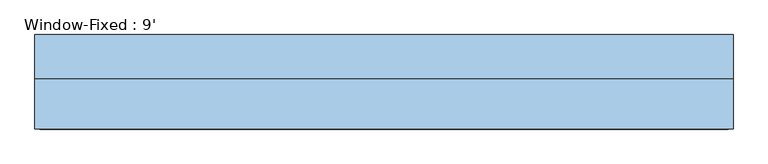
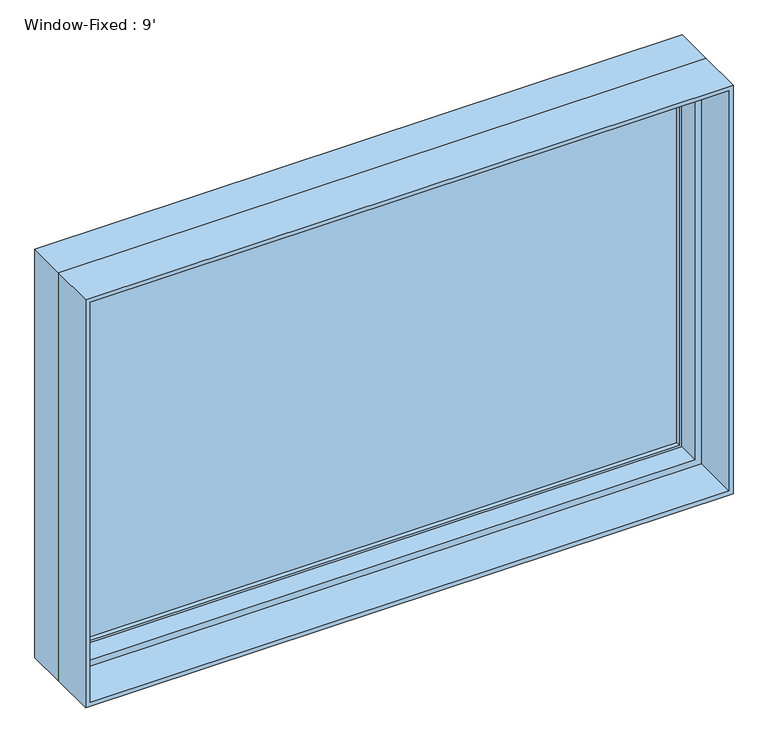
"""IFC4 building model written with IfcOpenShell, lengths in millimetres: window geometry, Window-Fixed : 9'."""

from ifc_helpers import new_model, si_unit, frame, origin, place, context, project, spatial, polyline, outline, extrude, faceted_brep, source, transform, mapped, element, save


def window_fixed_9_035f8342(model_context):
    return source(origin(), model_context, "Body", "SolidModel", [
        faceted_brep([(914.4, 19.05, 2133.6), (914.4, 133.35, 2133.6), (-914.4, 133.35, 2133.6), (-914.4, 19.05, 2133.6), (-914.4, 133.35, 914.4), (-914.4, 19.05, 914.4), (914.4, 133.35, 914.4), (914.4, 19.05, 914.4), (882.65, 19.05, 2101.85), (882.65, 19.05, 946.15), (-882.65, 19.05, 946.15), (-882.65, 19.05, 2101.85), (-901.7, 133.35, 2120.9), (-901.7, 133.35, 927.1), (901.7, 133.35, 927.1), (901.7, 133.35, 2120.9), (882.65, 82.55, 2101.85), (-882.65, 82.55, 2101.85), (901.7, 82.55, 2120.9), (-901.7, 82.55, 2120.9), (-882.65, 82.55, 946.15), (-901.7, 82.55, 927.1), (882.65, 82.55, 946.15), (901.7, 82.55, 927.1)], [[[0, 1, 2, 3]], [[3, 2, 4, 5]], [[5, 4, 6, 7]], [[3, 5, 7, 0], [8, 9, 10, 11]], [[7, 6, 1, 0]], [[1, 6, 4, 2], [12, 13, 14, 15]], [[16, 8, 11, 17]], [[15, 18, 19, 12]], [[17, 11, 10, 20]], [[12, 19, 21, 13]], [[20, 10, 9, 22]], [[13, 21, 23, 14]], [[22, 9, 8, 16]], [[18, 23, 21, 19], [17, 20, 22, 16]], [[14, 23, 18, 15]]]),
        extrude(outline(polyline([(2133.6, -914.4), (914.4, -914.4), (914.4, 914.4), (2133.6, 914.4), (2133.6, -914.4)]), holes=[polyline([(2120.9, 901.7), (927.1, 901.7), (927.1, -901.7), (2120.9, -901.7), (2120.9, 901.7)])]), frame((0.0, -114.3, 0.0), z_axis=(0.0, 1.0, 0.0), x_axis=(0.0, 0.0, 1.0)), (0.0, 0.0, 1.0), 133.35),
        extrude(outline(polyline([(927.1, 901.7), (2120.9, 901.7), (2120.9, -901.7), (927.1, -901.7), (927.1, 901.7)]), holes=[polyline([(952.5, -876.3), (2095.5, -876.3), (2095.5, 876.3), (952.5, 876.3), (952.5, -876.3)])]), frame((0.0, 82.55, 0.0), z_axis=(0.0, 1.0, 0.0), x_axis=(0.0, 0.0, 1.0)), (0.0, 0.0, 1.0), 44.45),
        extrude(outline(polyline([(876.3, 114.3), (876.3, 107.95), (-876.3, 107.95), (-876.3, 114.3), (876.3, 114.3)])), frame((0.0, 0.0, 952.5), z_axis=(0.0, 0.0, 1.0), x_axis=(1.0, 0.0, 0.0)), (0.0, 0.0, 1.0), 1143.0),
        extrude(outline(polyline([(-876.3, 95.25), (-876.3, 101.6), (876.3, 101.6), (876.3, 95.25), (-876.3, 95.25)])), frame((0.0, 0.0, 952.5), z_axis=(0.0, 0.0, 1.0), x_axis=(1.0, 0.0, 0.0)), (0.0, 0.0, 1.0), 1143.0),
    ])


if __name__ == "__main__":
    model = new_model("IFC4")
    model_context = context("Model", 3, world=origin())
    ifc_project = project(units=[si_unit("LENGTHUNIT", "METRE", prefix="MILLI")], contexts=[model_context])
    site = spatial("IfcSite", under=ifc_project)
    building = spatial("IfcBuilding", under=site)
    placement = place(None, origin())
    window_fixed_9_shape = window_fixed_9_035f8342(model_context)
    element("IfcWindow", 1, ObjectType="Window-Fixed : 9'", at=placement, inside=building, context=model_context, shape_type="MappedRepresentation", body=[
        mapped(window_fixed_9_shape, transform((0.0, 0.0, 0.0), x_axis=(1.0, 0.0, 0.0), y_axis=(0.0, 1.0, 0.0), z_axis=(0.0, 0.0, 1.0))),
    ])
    save(model, "model.ifc")

# Revit data of these elements
# Type "Window-Fixed : 9'"
#   Type Mark = "24"
#   Fire Rating = "0.5h"
#   Assembly Code = "B2020100"
#   Analytic Construction = "Double glazing - domestic"
#   Window Inset [instance default] = 0' - 0"
#   Wall Thickness [instance default] = 0' - 6"
#   Visual Light Transmittance = 0.81
#   Thermal Resistance (R) = 1.8146 (h·ft²·°F)/BTU
#   Solar Heat Gain Coefficient = 0.76
#   Rough Width = 6' - 0 1/2"
#   Rough Height = 4' - 0 1/2"
#   Interior Wall Closure [instance default] = 0' - 2 1/4"
#   Height = 4' - 0"
#   Heat Transfer Coefficient (U) = 0.5511 BTU/(h·ft²·°F)
#   Frame Extension [instance default] = 0' - 0 1/4"
#   Exterior Wall Closure [instance default] = 0' - 1 1/4"
#   Extension Jamb [instance default] = 0' - 2 1/4"
#   Default Sill Height = 3' - 0"
#   Width = 6' - 0"
#   Muntin Visibility = yes
#   Interior Trim Visibility [instance default] = yes
#   Exterior Trim Visibility [instance default] = yes
#   Extension Jamb Visibility [instance default] = yes
#   Muntin Pattern = Muntin Pattern_2x2 : Muntin Pattern_2x2
#   Interior Trim Material = Wood - Stained
#   Interior Trim = Trim-Window-Interior-Flat : Picture Frame
#   Interior Frame Material = Wood - Stained
#   Glass Panel Material = Glass
#   Exterior Trim Material = Clad - White
#   Exterior Trim = Trim-Window-Exterior-Flat : with Sill
#   Exterior Frame Material = Clad - White
#   Wall Closure = (empty or 0)
# Element 1 (IfcWindow, "Window-Fixed : 9'")
#   Wall Thickness = 0' - 9"
#   Extension Jamb = 0' - 5 1/4"
#   Materials on its faces: "Wood - Stained", "Glass", "Clad - White"
# Materials
#   "Wood - Stained": class "Wood", colour RGB 224 178 126, transparency 0, Cost = 0
#   "Glass": class "Glass", colour RGB 0 128 192, transparency 0.75, Description = "Soda Lime Glass", Cost = 0
#   "Clad - White": class "Wood", colour RGB 242 242 238, transparency 0, Cost = 0
